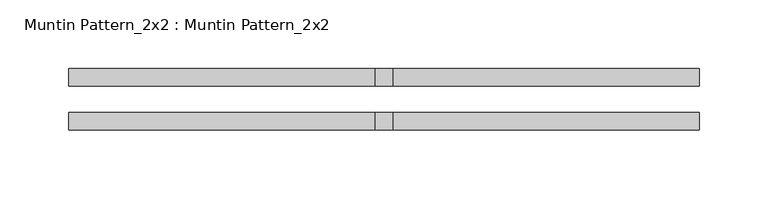
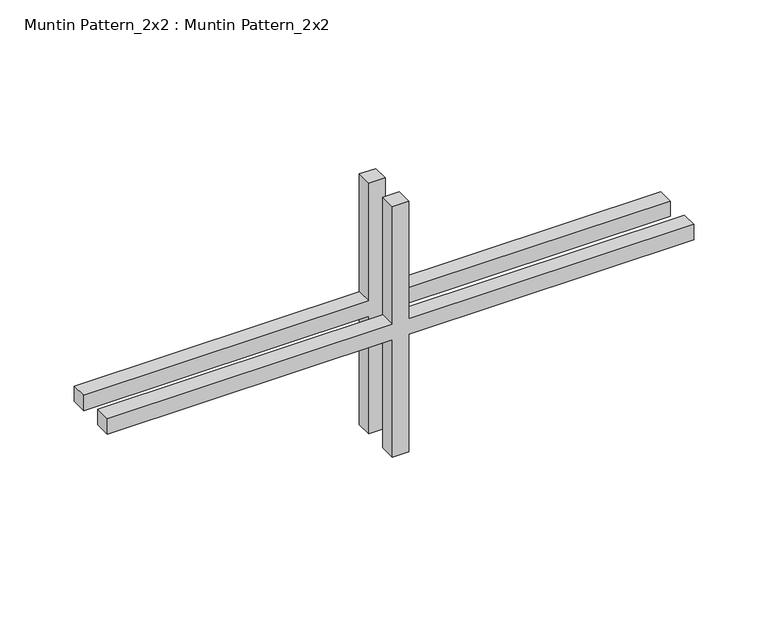
"""IFC4 building model written with IfcOpenShell, lengths in millimetres: proxy geometry, Muntin Pattern_2x2 : Muntin Pattern_2x2."""

from ifc_helpers import new_model, si_unit, frame, origin, place, context, project, spatial, polyline, outline, extrude, source, transform, mapped, element, save


def muntin_pattern_2x2_muntin_pattern_2x2_cfeb24ad(model_context):
    return source(origin(), model_context, "Body", "SweptSolid", [
        extrude(outline(polyline([(109.5375, -6.35), (109.5375, -228.6), (96.8375, -228.6), (96.8375, -6.35), (0.0, -6.35), (0.0, 6.35), (96.8375, 6.35), (96.8375, 228.6), (109.5375, 228.6), (109.5375, 6.35), (206.375, 6.35), (206.375, -6.35), (109.5375, -6.35)])), frame((0.0, 9.525, 0.0), z_axis=(0.0, 1.0, 0.0), x_axis=(0.0, 0.0, 1.0)), (0.0, 0.0, 1.0), 12.7),
        extrude(outline(polyline([(109.5375, -6.35), (109.5375, -228.6), (96.8375, -228.6), (96.8375, -6.35), (0.0, -6.35), (0.0, 6.35), (96.8375, 6.35), (96.8375, 228.6), (109.5375, 228.6), (109.5375, 6.35), (206.375, 6.35), (206.375, -6.35), (109.5375, -6.35)])), frame((0.0, -22.225, 0.0), z_axis=(0.0, 1.0, 0.0), x_axis=(0.0, 0.0, 1.0)), (0.0, 0.0, 1.0), 12.7),
    ])


if __name__ == "__main__":
    model = new_model("IFC4")
    model_context = context("Model", 3, world=origin())
    ifc_project = project(units=[si_unit("LENGTHUNIT", "METRE", prefix="MILLI")], contexts=[model_context])
    site = spatial("IfcSite", under=ifc_project)
    building = spatial("IfcBuilding", under=site)
    placement = place(None, origin())
    muntin_pattern_2x2_muntin_pattern_2x2_shape = muntin_pattern_2x2_muntin_pattern_2x2_cfeb24ad(model_context)
    element("IfcBuildingElementProxy", 1, Name="Muntin Pattern_2x2 : Muntin Pattern_2x2", ObjectType="Muntin Pattern_2x2 : Muntin Pattern_2x2", at=placement, inside=building, context=model_context, shape_type="MappedRepresentation", body=[
        mapped(muntin_pattern_2x2_muntin_pattern_2x2_shape, transform((0.0, 0.0, 0.0), x_axis=(1.0, 0.0, 0.0), y_axis=(0.0, 1.0, 0.0), z_axis=(0.0, 0.0, 1.0))),
    ])
    save(model, "model.ifc")

# Revit data of these elements
# Type "Muntin Pattern_2x2 : Muntin Pattern_2x2"
#   Width [instance default] = 4' - 0"
#   Thickness = 0' - 0 1/2"
#   Height [instance default] = 4' - 0"
#   Distance = 0' - 0 3/4"
#   Interior Material [instance default] = none
#   Exterior Material [instance default] = none
#   Default Elevation = 0
# Element 1 (IfcBuildingElementProxy, "Muntin Pattern_2x2 : Muntin Pattern_2x2")
#   Width = 1' - 6"
#   Height = 0' - 8 1/8"
#   Interior Material = Wood - Stained
#   Exterior Material = Clad - White
#   Materials on its faces: "Clad - White", "Wood - Stained"
# Materials
#   "Clad - White": class "Wood", colour RGB 242 242 238, transparency 0, Cost = 0
#   "Wood - Stained": class "Wood", colour RGB 224 178 126, transparency 0, Cost = 0
